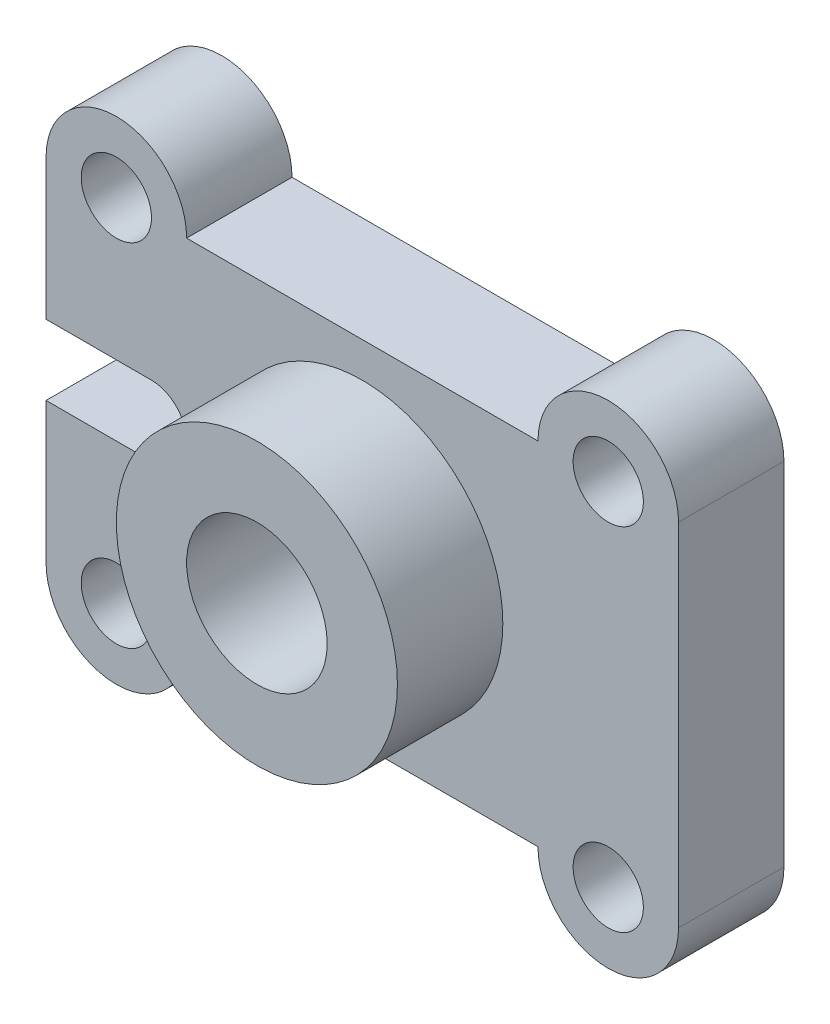
ISO-10303-21;
HEADER;
FILE_DESCRIPTION(('STEP AP214'),'2;1');
FILE_NAME('part.step','',(''),(''),'','','');
FILE_SCHEMA(('AUTOMOTIVE_DESIGN { 1 0 10303 214 1 1 1 1 }'));
ENDSEC;
DATA;
#1=APPLICATION_CONTEXT('core data for automotive mechanical design processes');
#2=APPLICATION_PROTOCOL_DEFINITION('international standard','automotive_design',2000,#1);
#3=PRODUCT_CONTEXT('',#1,'mechanical');
#4=PRODUCT('Part','Part','',(#3));
#5=PRODUCT_RELATED_PRODUCT_CATEGORY('part','',(#4));
#6=PRODUCT_DEFINITION_FORMATION('','',#4);
#7=PRODUCT_DEFINITION_CONTEXT('part definition',#1,'design');
#8=PRODUCT_DEFINITION('design','',#6,#7);
#9=PRODUCT_DEFINITION_SHAPE('','',#8);
#10=(LENGTH_UNIT() NAMED_UNIT(*) SI_UNIT(.MILLI.,.METRE.));
#11=(NAMED_UNIT(*) PLANE_ANGLE_UNIT() SI_UNIT($,.RADIAN.));
#12=(NAMED_UNIT(*) SI_UNIT($,.STERADIAN.) SOLID_ANGLE_UNIT());
#13=UNCERTAINTY_MEASURE_WITH_UNIT(LENGTH_MEASURE(1.E-05),#10,'distance_accuracy_value','');
#14=(GEOMETRIC_REPRESENTATION_CONTEXT(3) GLOBAL_UNCERTAINTY_ASSIGNED_CONTEXT((#13)) GLOBAL_UNIT_ASSIGNED_CONTEXT((#10,
#11,#12)) REPRESENTATION_CONTEXT('',''));
#15=CARTESIAN_POINT('',(0.,0.,0.));
#16=DIRECTION('',(0.,0.,1.));
#17=DIRECTION('',(1.,0.,0.));
#18=AXIS2_PLACEMENT_3D('',#15,#16,#17);
#19=CARTESIAN_POINT('',(8.92547525553978E-07,-50.0000066960144,15.));
#20=DIRECTION('',(0.,0.,-1.));
#21=DIRECTION('',(-1.,0.,0.));
#22=AXIS2_PLACEMENT_3D('',#19,#20,#21);
#23=CYLINDRICAL_SURFACE('',#22,10.0000000000001);
#24=CARTESIAN_POINT('',(8.92547525553978E-07,-50.0000066960144,0.));
#25=DIRECTION('',(0.,0.,1.));
#26=DIRECTION('',(1.,0.,0.));
#27=AXIS2_PLACEMENT_3D('',#24,#25,#26);
#28=CIRCLE('',#27,10.0000000000001);
#29=CARTESIAN_POINT('',(-9.99999910745245,-50.0000066960144,0.));
#30=VERTEX_POINT('',#29);
#31=CARTESIAN_POINT('',(10.0000008925476,-50.0000051331027,0.));
#32=VERTEX_POINT('',#31);
#33=EDGE_CURVE('E164',#30,#32,#28,.T.);
#34=ORIENTED_EDGE('',*,*,#33,.T.);
#35=DIRECTION('',(0.,0.,-1.));
#36=VECTOR('',#35,1.);
#37=CARTESIAN_POINT('',(10.0000008925476,-50.0000051331027,15.));
#38=LINE('',#37,#36);
#39=CARTESIAN_POINT('',(10.0000008925476,-50.0000051331027,15.));
#40=VERTEX_POINT('',#39);
#41=EDGE_CURVE('E11',#40,#32,#38,.T.);
#42=ORIENTED_EDGE('',*,*,#41,.F.);
#43=CARTESIAN_POINT('',(8.92547525553978E-07,-50.0000066960144,15.));
#44=DIRECTION('',(0.,0.,1.));
#45=DIRECTION('',(1.,0.,0.));
#46=AXIS2_PLACEMENT_3D('',#43,#44,#45);
#47=CIRCLE('',#46,10.0000000000001);
#48=CARTESIAN_POINT('',(-9.99999910745245,-50.0000066960144,15.));
#49=VERTEX_POINT('',#48);
#50=EDGE_CURVE('E186',#49,#40,#47,.T.);
#51=ORIENTED_EDGE('',*,*,#50,.F.);
#52=DIRECTION('',(0.,0.,-1.));
#53=VECTOR('',#52,1.);
#54=CARTESIAN_POINT('',(-9.99999910745245,-50.0000066960144,15.));
#55=LINE('',#54,#53);
#56=EDGE_CURVE('E161',#49,#30,#55,.T.);
#57=ORIENTED_EDGE('',*,*,#56,.T.);
#58=EDGE_LOOP('',(#34,#42,#51,#57));
#59=FACE_BOUND('',#58,.T.);
#60=ADVANCED_FACE('F44',(#59),#23,.T.);
#61=CARTESIAN_POINT('',(59.9999991074522,-50.0000051331027,15.));
#62=DIRECTION('',(0.,1.,0.));
#63=DIRECTION('',(-1.,0.,0.));
#64=AXIS2_PLACEMENT_3D('',#61,#62,#63);
#65=PLANE('',#64);
#66=DIRECTION('',(1.,0.,0.));
#67=VECTOR('',#66,1.);
#68=CARTESIAN_POINT('',(59.9999991074522,-50.0000051331027,0.));
#69=LINE('',#68,#67);
#70=CARTESIAN_POINT('',(59.9999991074522,-50.0000051331027,0.));
#71=VERTEX_POINT('',#70);
#72=EDGE_CURVE('E169',#32,#71,#69,.T.);
#73=ORIENTED_EDGE('',*,*,#72,.T.);
#74=DIRECTION('',(0.,0.,-1.));
#75=VECTOR('',#74,1.);
#76=CARTESIAN_POINT('',(59.9999991074522,-50.0000051331027,15.));
#77=LINE('',#76,#75);
#78=CARTESIAN_POINT('',(59.9999991074522,-50.0000051331027,15.));
#79=VERTEX_POINT('',#78);
#80=EDGE_CURVE('E52',#79,#71,#77,.T.);
#81=ORIENTED_EDGE('',*,*,#80,.F.);
#82=DIRECTION('',(1.,0.,0.));
#83=VECTOR('',#82,1.);
#84=CARTESIAN_POINT('',(59.9999991074522,-50.0000051331027,15.));
#85=LINE('',#84,#83);
#86=EDGE_CURVE('E118',#40,#79,#85,.T.);
#87=ORIENTED_EDGE('',*,*,#86,.F.);
#88=ORIENTED_EDGE('',*,*,#41,.T.);
#89=EDGE_LOOP('',(#73,#81,#87,#88));
#90=FACE_BOUND('',#89,.T.);
#91=ADVANCED_FACE('F267',(#90),#65,.F.);
#92=CARTESIAN_POINT('',(69.9999991074519,-50.0000000000001,15.));
#93=DIRECTION('',(0.,0.,-1.));
#94=DIRECTION('',(-1.,0.,0.));
#95=AXIS2_PLACEMENT_3D('',#92,#93,#94);
#96=CYLINDRICAL_SURFACE('',#95,10.0000000000006);
#97=CARTESIAN_POINT('',(69.9999991074519,-50.0000000000001,0.));
#98=DIRECTION('',(0.,0.,1.));
#99=DIRECTION('',(1.,0.,0.));
#100=AXIS2_PLACEMENT_3D('',#97,#98,#99);
#101=CIRCLE('',#100,10.0000000000006);
#102=CARTESIAN_POINT('',(79.9999991074525,-50.0000000000001,0.));
#103=VERTEX_POINT('',#102);
#104=EDGE_CURVE('E173',#71,#103,#101,.T.);
#105=ORIENTED_EDGE('',*,*,#104,.T.);
#106=DIRECTION('',(0.,0.,-1.));
#107=VECTOR('',#106,1.);
#108=CARTESIAN_POINT('',(79.9999991074525,-50.0000000000001,15.));
#109=LINE('',#108,#107);
#110=CARTESIAN_POINT('',(79.9999991074525,-50.0000000000001,15.));
#111=VERTEX_POINT('',#110);
#112=EDGE_CURVE('E210',#111,#103,#109,.T.);
#113=ORIENTED_EDGE('',*,*,#112,.F.);
#114=CARTESIAN_POINT('',(69.9999991074519,-50.0000000000001,15.));
#115=DIRECTION('',(0.,0.,1.));
#116=DIRECTION('',(1.,0.,0.));
#117=AXIS2_PLACEMENT_3D('',#114,#115,#116);
#118=CIRCLE('',#117,10.0000000000006);
#119=EDGE_CURVE('E214',#79,#111,#118,.T.);
#120=ORIENTED_EDGE('',*,*,#119,.F.);
#121=ORIENTED_EDGE('',*,*,#80,.T.);
#122=EDGE_LOOP('',(#105,#113,#120,#121));
#123=FACE_BOUND('',#122,.T.);
#124=ADVANCED_FACE('F213',(#123),#96,.T.);
#125=CARTESIAN_POINT('',(79.999999107452,0.,15.));
#126=DIRECTION('',(-1.,0.,0.));
#127=DIRECTION('',(0.,-1.,0.));
#128=AXIS2_PLACEMENT_3D('',#125,#126,#127);
#129=PLANE('',#128);
#130=DIRECTION('',(0.,1.,0.));
#131=VECTOR('',#130,1.);
#132=CARTESIAN_POINT('',(79.999999107452,0.,0.));
#133=LINE('',#132,#131);
#134=CARTESIAN_POINT('',(79.999999107452,0.,0.));
#135=VERTEX_POINT('',#134);
#136=EDGE_CURVE('E171',#103,#135,#133,.T.);
#137=ORIENTED_EDGE('',*,*,#136,.T.);
#138=DIRECTION('',(0.,0.,-1.));
#139=VECTOR('',#138,1.);
#140=CARTESIAN_POINT('',(79.999999107452,0.,15.));
#141=LINE('',#140,#139);
#142=CARTESIAN_POINT('',(79.999999107452,0.,15.));
#143=VERTEX_POINT('',#142);
#144=EDGE_CURVE('E204',#143,#135,#141,.T.);
#145=ORIENTED_EDGE('',*,*,#144,.F.);
#146=DIRECTION('',(0.,1.,0.));
#147=VECTOR('',#146,1.);
#148=CARTESIAN_POINT('',(79.999999107452,0.,15.));
#149=LINE('',#148,#147);
#150=EDGE_CURVE('E235',#111,#143,#149,.T.);
#151=ORIENTED_EDGE('',*,*,#150,.F.);
#152=ORIENTED_EDGE('',*,*,#112,.T.);
#153=EDGE_LOOP('',(#137,#145,#151,#152));
#154=FACE_BOUND('',#153,.T.);
#155=ADVANCED_FACE('F221',(#154),#129,.F.);
#156=CARTESIAN_POINT('',(69.999999107452,0.,15.));
#157=DIRECTION('',(0.,0.,-1.));
#158=DIRECTION('',(-1.,0.,0.));
#159=AXIS2_PLACEMENT_3D('',#156,#157,#158);
#160=CYLINDRICAL_SURFACE('',#159,10.0000000000005);
#161=CARTESIAN_POINT('',(69.999999107452,0.,0.));
#162=DIRECTION('',(0.,0.,1.));
#163=DIRECTION('',(1.,0.,0.));
#164=AXIS2_PLACEMENT_3D('',#161,#162,#163);
#165=CIRCLE('',#164,10.0000000000005);
#166=CARTESIAN_POINT('',(59.9999991074528,-5.13310270243646E-06,0.));
#167=VERTEX_POINT('',#166);
#168=EDGE_CURVE('E172',#135,#167,#165,.T.);
#169=ORIENTED_EDGE('',*,*,#168,.T.);
#170=DIRECTION('',(0.,0.,-1.));
#171=VECTOR('',#170,1.);
#172=CARTESIAN_POINT('',(59.9999991074528,-5.13310270243646E-06,15.));
#173=LINE('',#172,#171);
#174=CARTESIAN_POINT('',(59.9999991074528,-5.13310270243646E-06,15.));
#175=VERTEX_POINT('',#174);
#176=EDGE_CURVE('E203',#175,#167,#173,.T.);
#177=ORIENTED_EDGE('',*,*,#176,.F.);
#178=CARTESIAN_POINT('',(69.999999107452,0.,15.));
#179=DIRECTION('',(0.,0.,1.));
#180=DIRECTION('',(1.,0.,0.));
#181=AXIS2_PLACEMENT_3D('',#178,#179,#180);
#182=CIRCLE('',#181,10.0000000000005);
#183=EDGE_CURVE('E227',#143,#175,#182,.T.);
#184=ORIENTED_EDGE('',*,*,#183,.F.);
#185=ORIENTED_EDGE('',*,*,#144,.T.);
#186=EDGE_LOOP('',(#169,#177,#184,#185));
#187=FACE_BOUND('',#186,.T.);
#188=ADVANCED_FACE('F226',(#187),#160,.T.);
#189=CARTESIAN_POINT('',(9.99999910745228,-5.13310270598176E-06,15.));
#190=DIRECTION('',(0.,-1.,0.));
#191=DIRECTION('',(1.,0.,0.));
#192=AXIS2_PLACEMENT_3D('',#189,#190,#191);
#193=PLANE('',#192);
#194=DIRECTION('',(-1.,0.,0.));
#195=VECTOR('',#194,1.);
#196=CARTESIAN_POINT('',(9.99999910745228,-5.13310270598176E-06,0.));
#197=LINE('',#196,#195);
#198=CARTESIAN_POINT('',(9.99999910745228,-5.13310270598176E-06,0.));
#199=VERTEX_POINT('',#198);
#200=EDGE_CURVE('E179',#167,#199,#197,.T.);
#201=ORIENTED_EDGE('',*,*,#200,.T.);
#202=DIRECTION('',(0.,0.,-1.));
#203=VECTOR('',#202,1.);
#204=CARTESIAN_POINT('',(9.99999910745228,-5.13310270598176E-06,15.));
#205=LINE('',#204,#203);
#206=CARTESIAN_POINT('',(9.99999910745228,-5.13310270598176E-06,15.));
#207=VERTEX_POINT('',#206);
#208=EDGE_CURVE('E196',#207,#199,#205,.T.);
#209=ORIENTED_EDGE('',*,*,#208,.F.);
#210=DIRECTION('',(-1.,0.,0.));
#211=VECTOR('',#210,1.);
#212=CARTESIAN_POINT('',(9.99999910745228,-5.13310270598176E-06,15.));
#213=LINE('',#212,#211);
#214=EDGE_CURVE('E234',#175,#207,#213,.T.);
#215=ORIENTED_EDGE('',*,*,#214,.F.);
#216=ORIENTED_EDGE('',*,*,#176,.T.);
#217=EDGE_LOOP('',(#201,#209,#215,#216));
#218=FACE_BOUND('',#217,.T.);
#219=ADVANCED_FACE('F284',(#218),#193,.F.);
#220=CARTESIAN_POINT('',(0.,0.,15.));
#221=DIRECTION('',(0.,0.,-1.));
#222=DIRECTION('',(-1.,0.,0.));
#223=AXIS2_PLACEMENT_3D('',#220,#221,#222);
#224=CYLINDRICAL_SURFACE('',#223,9.99999910745303);
#225=CARTESIAN_POINT('',(0.,0.,0.));
#226=DIRECTION('',(0.,0.,1.));
#227=DIRECTION('',(1.,0.,0.));
#228=AXIS2_PLACEMENT_3D('',#225,#226,#227);
#229=CIRCLE('',#228,9.99999910745303);
#230=CARTESIAN_POINT('',(-9.99999910745303,0.,0.));
#231=VERTEX_POINT('',#230);
#232=EDGE_CURVE('E176',#199,#231,#229,.T.);
#233=ORIENTED_EDGE('',*,*,#232,.T.);
#234=DIRECTION('',(0.,0.,-1.));
#235=VECTOR('',#234,1.);
#236=CARTESIAN_POINT('',(-9.99999910745303,0.,15.));
#237=LINE('',#236,#235);
#238=CARTESIAN_POINT('',(-9.99999910745303,0.,15.));
#239=VERTEX_POINT('',#238);
#240=EDGE_CURVE('E193',#239,#231,#237,.T.);
#241=ORIENTED_EDGE('',*,*,#240,.F.);
#242=CARTESIAN_POINT('',(0.,0.,15.));
#243=DIRECTION('',(0.,0.,1.));
#244=DIRECTION('',(1.,0.,0.));
#245=AXIS2_PLACEMENT_3D('',#242,#243,#244);
#246=CIRCLE('',#245,9.99999910745303);
#247=EDGE_CURVE('E233',#207,#239,#246,.T.);
#248=ORIENTED_EDGE('',*,*,#247,.F.);
#249=ORIENTED_EDGE('',*,*,#208,.T.);
#250=EDGE_LOOP('',(#233,#241,#248,#249));
#251=FACE_BOUND('',#250,.T.);
#252=ADVANCED_FACE('F289',(#251),#224,.T.);
#253=CARTESIAN_POINT('',(-9.99999910745246,0.,15.));
#254=DIRECTION('',(1.,0.,0.));
#255=DIRECTION('',(0.,1.,0.));
#256=AXIS2_PLACEMENT_3D('',#253,#254,#255);
#257=PLANE('',#256);
#258=DIRECTION('',(0.,-1.,0.));
#259=VECTOR('',#258,1.);
#260=CARTESIAN_POINT('',(-9.99999910745246,0.,0.));
#261=LINE('',#260,#259);
#262=CARTESIAN_POINT('',(-9.99999910745245,-20.,0.));
#263=VERTEX_POINT('',#262);
#264=EDGE_CURVE('E182',#231,#263,#261,.T.);
#265=ORIENTED_EDGE('',*,*,#264,.T.);
#266=DIRECTION('',(0.,0.,-1.));
#267=VECTOR('',#266,1.);
#268=CARTESIAN_POINT('',(-9.99999910745245,-20.,15.));
#269=LINE('',#268,#267);
#270=CARTESIAN_POINT('',(-9.99999910745245,-20.,15.));
#271=VERTEX_POINT('',#270);
#272=EDGE_CURVE('E194',#271,#263,#269,.T.);
#273=ORIENTED_EDGE('',*,*,#272,.F.);
#274=DIRECTION('',(0.,-1.,0.));
#275=VECTOR('',#274,1.);
#276=CARTESIAN_POINT('',(-9.99999910745246,0.,15.));
#277=LINE('',#276,#275);
#278=EDGE_CURVE('E243',#239,#271,#277,.T.);
#279=ORIENTED_EDGE('',*,*,#278,.F.);
#280=ORIENTED_EDGE('',*,*,#240,.T.);
#281=EDGE_LOOP('',(#265,#273,#279,#280));
#282=FACE_BOUND('',#281,.T.);
#283=ADVANCED_FACE('F249',(#282),#257,.F.);
#284=CARTESIAN_POINT('',(-9.99999910745245,-20.,15.));
#285=DIRECTION('',(0.,1.,0.));
#286=DIRECTION('',(-1.,0.,0.));
#287=AXIS2_PLACEMENT_3D('',#284,#285,#286);
#288=PLANE('',#287);
#289=DIRECTION('',(1.,0.,0.));
#290=VECTOR('',#289,1.);
#291=CARTESIAN_POINT('',(-9.99999910745245,-20.,0.));
#292=LINE('',#291,#290);
#293=CARTESIAN_POINT('',(5.00000267764276,-20.,0.));
#294=VERTEX_POINT('',#293);
#295=EDGE_CURVE('E181',#263,#294,#292,.T.);
#296=ORIENTED_EDGE('',*,*,#295,.T.);
#297=DIRECTION('',(0.,0.,-1.));
#298=VECTOR('',#297,1.);
#299=CARTESIAN_POINT('',(5.00000267764276,-20.,15.));
#300=LINE('',#299,#298);
#301=CARTESIAN_POINT('',(5.00000267764276,-20.,15.));
#302=VERTEX_POINT('',#301);
#303=EDGE_CURVE('E156',#302,#294,#300,.T.);
#304=ORIENTED_EDGE('',*,*,#303,.F.);
#305=DIRECTION('',(1.,0.,0.));
#306=VECTOR('',#305,1.);
#307=CARTESIAN_POINT('',(-9.99999910745245,-20.,15.));
#308=LINE('',#307,#306);
#309=EDGE_CURVE('E150',#271,#302,#308,.T.);
#310=ORIENTED_EDGE('',*,*,#309,.F.);
#311=ORIENTED_EDGE('',*,*,#272,.T.);
#312=EDGE_LOOP('',(#296,#304,#310,#311));
#313=FACE_BOUND('',#312,.T.);
#314=ADVANCED_FACE('F253',(#313),#288,.F.);
#315=CARTESIAN_POINT('',(5.00000169147834,-25.,15.));
#316=DIRECTION('',(0.,0.,-1.));
#317=DIRECTION('',(-1.,0.,0.));
#318=AXIS2_PLACEMENT_3D('',#315,#316,#317);
#319=CYLINDRICAL_SURFACE('',#318,5.00000000000008);
#320=CARTESIAN_POINT('',(5.00000169147834,-25.,0.));
#321=DIRECTION('',(0.,0.,-1.));
#322=DIRECTION('',(1.,0.,0.));
#323=AXIS2_PLACEMENT_3D('',#320,#321,#322);
#324=CIRCLE('',#323,5.00000000000008);
#325=CARTESIAN_POINT('',(5.00000089254754,-30.0000000000001,0.));
#326=VERTEX_POINT('',#325);
#327=EDGE_CURVE('E154',#294,#326,#324,.T.);
#328=ORIENTED_EDGE('',*,*,#327,.T.);
#329=DIRECTION('',(0.,0.,-1.));
#330=VECTOR('',#329,1.);
#331=CARTESIAN_POINT('',(5.00000089254754,-30.0000000000001,15.));
#332=LINE('',#331,#330);
#333=CARTESIAN_POINT('',(5.00000089254754,-30.0000000000001,15.));
#334=VERTEX_POINT('',#333);
#335=EDGE_CURVE('E155',#334,#326,#332,.T.);
#336=ORIENTED_EDGE('',*,*,#335,.F.);
#337=CARTESIAN_POINT('',(5.00000169147834,-25.,15.));
#338=DIRECTION('',(0.,0.,-1.));
#339=DIRECTION('',(1.,0.,0.));
#340=AXIS2_PLACEMENT_3D('',#337,#338,#339);
#341=CIRCLE('',#340,5.00000000000008);
#342=EDGE_CURVE('E143',#302,#334,#341,.T.);
#343=ORIENTED_EDGE('',*,*,#342,.F.);
#344=ORIENTED_EDGE('',*,*,#303,.T.);
#345=EDGE_LOOP('',(#328,#336,#343,#344));
#346=FACE_BOUND('',#345,.T.);
#347=ADVANCED_FACE('F153',(#346),#319,.F.);
#348=CARTESIAN_POINT('',(5.00000089254754,-30.,15.));
#349=DIRECTION('',(0.,-1.,0.));
#350=DIRECTION('',(1.,0.,0.));
#351=AXIS2_PLACEMENT_3D('',#348,#349,#350);
#352=PLANE('',#351);
#353=DIRECTION('',(-1.,0.,0.));
#354=VECTOR('',#353,1.);
#355=CARTESIAN_POINT('',(5.00000089254754,-30.,0.));
#356=LINE('',#355,#354);
#357=CARTESIAN_POINT('',(-9.99999910745245,-30.,0.));
#358=VERTEX_POINT('',#357);
#359=EDGE_CURVE('E105',#326,#358,#356,.T.);
#360=ORIENTED_EDGE('',*,*,#359,.T.);
#361=DIRECTION('',(0.,0.,-1.));
#362=VECTOR('',#361,1.);
#363=CARTESIAN_POINT('',(-9.99999910745245,-30.,15.));
#364=LINE('',#363,#362);
#365=CARTESIAN_POINT('',(-9.99999910745245,-30.,15.));
#366=VERTEX_POINT('',#365);
#367=EDGE_CURVE('E160',#366,#358,#364,.T.);
#368=ORIENTED_EDGE('',*,*,#367,.F.);
#369=DIRECTION('',(-1.,0.,0.));
#370=VECTOR('',#369,1.);
#371=CARTESIAN_POINT('',(5.00000089254754,-30.,15.));
#372=LINE('',#371,#370);
#373=EDGE_CURVE('E144',#334,#366,#372,.T.);
#374=ORIENTED_EDGE('',*,*,#373,.F.);
#375=ORIENTED_EDGE('',*,*,#335,.T.);
#376=EDGE_LOOP('',(#360,#368,#374,#375));
#377=FACE_BOUND('',#376,.T.);
#378=ADVANCED_FACE('F157',(#377),#352,.F.);
#379=CARTESIAN_POINT('',(-9.99999910745245,-30.,15.));
#380=DIRECTION('',(1.,0.,0.));
#381=DIRECTION('',(0.,1.,0.));
#382=AXIS2_PLACEMENT_3D('',#379,#380,#381);
#383=PLANE('',#382);
#384=DIRECTION('',(0.,-1.,0.));
#385=VECTOR('',#384,1.);
#386=CARTESIAN_POINT('',(-9.99999910745245,-30.,0.));
#387=LINE('',#386,#385);
#388=EDGE_CURVE('E107',#358,#30,#387,.T.);
#389=ORIENTED_EDGE('',*,*,#388,.T.);
#390=ORIENTED_EDGE('',*,*,#56,.F.);
#391=DIRECTION('',(0.,-1.,0.));
#392=VECTOR('',#391,1.);
#393=CARTESIAN_POINT('',(-9.99999910745245,-30.,15.));
#394=LINE('',#393,#392);
#395=EDGE_CURVE('E63',#366,#49,#394,.T.);
#396=ORIENTED_EDGE('',*,*,#395,.F.);
#397=ORIENTED_EDGE('',*,*,#367,.T.);
#398=EDGE_LOOP('',(#389,#390,#396,#397));
#399=FACE_BOUND('',#398,.T.);
#400=ADVANCED_FACE('F254',(#399),#383,.F.);
#401=CARTESIAN_POINT('',(8.92547525553978E-07,-50.0000066960144,15.));
#402=DIRECTION('',(0.,0.,1.));
#403=DIRECTION('',(1.,0.,0.));
#404=AXIS2_PLACEMENT_3D('',#401,#402,#403);
#405=PLANE('',#404);
#406=CARTESIAN_POINT('',(34.9999991074525,-25.0000051331027,15.));
#407=DIRECTION('',(0.,0.,1.));
#408=DIRECTION('',(1.,0.,0.));
#409=AXIS2_PLACEMENT_3D('',#406,#407,#408);
#410=CIRCLE('',#409,20.);
#411=CARTESIAN_POINT('',(54.9999991074525,-25.0000051331027,15.));
#412=VERTEX_POINT('',#411);
#413=EDGE_CURVE('E567',#412,#412,#410,.T.);
#414=ORIENTED_EDGE('',*,*,#413,.F.);
#415=EDGE_LOOP('',(#414));
#416=FACE_BOUND('',#415,.T.);
#417=CARTESIAN_POINT('',(8.92547525553978E-07,-50.0000066960144,15.));
#418=DIRECTION('',(0.,0.,1.));
#419=DIRECTION('',(1.,0.,0.));
#420=AXIS2_PLACEMENT_3D('',#417,#418,#419);
#421=CIRCLE('',#420,5.00000000000001);
#422=CARTESIAN_POINT('',(5.00000089254753,-50.0000066960144,15.));
#423=VERTEX_POINT('',#422);
#424=EDGE_CURVE('E552',#423,#423,#421,.T.);
#425=ORIENTED_EDGE('',*,*,#424,.F.);
#426=EDGE_LOOP('',(#425));
#427=FACE_BOUND('',#426,.T.);
#428=CARTESIAN_POINT('',(69.9999991074519,-50.0000000000001,15.));
#429=DIRECTION('',(0.,0.,1.));
#430=DIRECTION('',(1.,0.,0.));
#431=AXIS2_PLACEMENT_3D('',#428,#429,#430);
#432=CIRCLE('',#431,5.00000000000001);
#433=CARTESIAN_POINT('',(74.9999991074519,-50.0000000000001,15.));
#434=VERTEX_POINT('',#433);
#435=EDGE_CURVE('E556',#434,#434,#432,.T.);
#436=ORIENTED_EDGE('',*,*,#435,.F.);
#437=EDGE_LOOP('',(#436));
#438=FACE_BOUND('',#437,.T.);
#439=CARTESIAN_POINT('',(69.999999107452,0.,15.));
#440=DIRECTION('',(0.,0.,1.));
#441=DIRECTION('',(1.,0.,0.));
#442=AXIS2_PLACEMENT_3D('',#439,#440,#441);
#443=CIRCLE('',#442,5.);
#444=CARTESIAN_POINT('',(74.999999107452,0.,15.));
#445=VERTEX_POINT('',#444);
#446=EDGE_CURVE('E564',#445,#445,#443,.T.);
#447=ORIENTED_EDGE('',*,*,#446,.F.);
#448=EDGE_LOOP('',(#447));
#449=FACE_BOUND('',#448,.T.);
#450=CARTESIAN_POINT('',(0.,0.,15.));
#451=DIRECTION('',(0.,0.,1.));
#452=DIRECTION('',(1.,0.,0.));
#453=AXIS2_PLACEMENT_3D('',#450,#451,#452);
#454=CIRCLE('',#453,5.);
#455=CARTESIAN_POINT('',(5.,0.,15.));
#456=VERTEX_POINT('',#455);
#457=EDGE_CURVE('E546',#456,#456,#454,.T.);
#458=ORIENTED_EDGE('',*,*,#457,.F.);
#459=EDGE_LOOP('',(#458));
#460=FACE_BOUND('',#459,.T.);
#461=ORIENTED_EDGE('',*,*,#50,.T.);
#462=ORIENTED_EDGE('',*,*,#86,.T.);
#463=ORIENTED_EDGE('',*,*,#119,.T.);
#464=ORIENTED_EDGE('',*,*,#150,.T.);
#465=ORIENTED_EDGE('',*,*,#183,.T.);
#466=ORIENTED_EDGE('',*,*,#214,.T.);
#467=ORIENTED_EDGE('',*,*,#247,.T.);
#468=ORIENTED_EDGE('',*,*,#278,.T.);
#469=ORIENTED_EDGE('',*,*,#309,.T.);
#470=ORIENTED_EDGE('',*,*,#342,.T.);
#471=ORIENTED_EDGE('',*,*,#373,.T.);
#472=ORIENTED_EDGE('',*,*,#395,.T.);
#473=EDGE_LOOP('',(#461,#462,#463,#464,#465,#466,#467,#468,#469,#470,#471,#472));
#474=FACE_BOUND('',#473,.T.);
#475=ADVANCED_FACE('F141',(#416,#427,#438,#449,#460,#474),#405,.T.);
#476=CARTESIAN_POINT('',(8.92547525553978E-07,-50.0000066960144,0.));
#477=DIRECTION('',(0.,0.,1.));
#478=DIRECTION('',(1.,0.,0.));
#479=AXIS2_PLACEMENT_3D('',#476,#477,#478);
#480=PLANE('',#479);
#481=CARTESIAN_POINT('',(8.92547525553978E-07,-50.0000066960144,0.));
#482=DIRECTION('',(0.,0.,1.));
#483=DIRECTION('',(1.,0.,0.));
#484=AXIS2_PLACEMENT_3D('',#481,#482,#483);
#485=CIRCLE('',#484,5.00000000000001);
#486=CARTESIAN_POINT('',(5.00000089254753,-50.0000066960144,0.));
#487=VERTEX_POINT('',#486);
#488=EDGE_CURVE('E532',#487,#487,#485,.T.);
#489=ORIENTED_EDGE('',*,*,#488,.T.);
#490=EDGE_LOOP('',(#489));
#491=FACE_BOUND('',#490,.T.);
#492=CARTESIAN_POINT('',(69.9999991074519,-50.0000000000001,0.));
#493=DIRECTION('',(0.,0.,1.));
#494=DIRECTION('',(1.,0.,0.));
#495=AXIS2_PLACEMENT_3D('',#492,#493,#494);
#496=CIRCLE('',#495,5.00000000000001);
#497=CARTESIAN_POINT('',(74.9999991074519,-50.0000000000001,0.));
#498=VERTEX_POINT('',#497);
#499=EDGE_CURVE('E537',#498,#498,#496,.T.);
#500=ORIENTED_EDGE('',*,*,#499,.T.);
#501=EDGE_LOOP('',(#500));
#502=FACE_BOUND('',#501,.T.);
#503=CARTESIAN_POINT('',(69.999999107452,0.,0.));
#504=DIRECTION('',(0.,0.,1.));
#505=DIRECTION('',(1.,0.,0.));
#506=AXIS2_PLACEMENT_3D('',#503,#504,#505);
#507=CIRCLE('',#506,5.);
#508=CARTESIAN_POINT('',(74.999999107452,0.,0.));
#509=VERTEX_POINT('',#508);
#510=EDGE_CURVE('E543',#509,#509,#507,.T.);
#511=ORIENTED_EDGE('',*,*,#510,.T.);
#512=EDGE_LOOP('',(#511));
#513=FACE_BOUND('',#512,.T.);
#514=CARTESIAN_POINT('',(0.,0.,0.));
#515=DIRECTION('',(0.,0.,1.));
#516=DIRECTION('',(1.,0.,0.));
#517=AXIS2_PLACEMENT_3D('',#514,#515,#516);
#518=CIRCLE('',#517,5.);
#519=CARTESIAN_POINT('',(5.,0.,0.));
#520=VERTEX_POINT('',#519);
#521=EDGE_CURVE('E166',#520,#520,#518,.T.);
#522=ORIENTED_EDGE('',*,*,#521,.T.);
#523=EDGE_LOOP('',(#522));
#524=FACE_BOUND('',#523,.T.);
#525=ORIENTED_EDGE('',*,*,#33,.F.);
#526=ORIENTED_EDGE('',*,*,#388,.F.);
#527=ORIENTED_EDGE('',*,*,#359,.F.);
#528=ORIENTED_EDGE('',*,*,#327,.F.);
#529=ORIENTED_EDGE('',*,*,#295,.F.);
#530=ORIENTED_EDGE('',*,*,#264,.F.);
#531=ORIENTED_EDGE('',*,*,#232,.F.);
#532=ORIENTED_EDGE('',*,*,#200,.F.);
#533=ORIENTED_EDGE('',*,*,#168,.F.);
#534=ORIENTED_EDGE('',*,*,#136,.F.);
#535=ORIENTED_EDGE('',*,*,#104,.F.);
#536=ORIENTED_EDGE('',*,*,#72,.F.);
#537=EDGE_LOOP('',(#525,#526,#527,#528,#529,#530,#531,#532,#533,#534,#535,#536));
#538=FACE_BOUND('',#537,.T.);
#539=ADVANCED_FACE('F218',(#491,#502,#513,#524,#538),#480,.F.);
#540=CARTESIAN_POINT('',(0.,0.,0.));
#541=DIRECTION('',(0.,0.,1.));
#542=DIRECTION('',(1.,0.,0.));
#543=AXIS2_PLACEMENT_3D('',#540,#541,#542);
#544=CYLINDRICAL_SURFACE('',#543,5.);
#545=ORIENTED_EDGE('',*,*,#521,.F.);
#546=EDGE_LOOP('',(#545));
#547=FACE_BOUND('',#546,.T.);
#548=ORIENTED_EDGE('',*,*,#457,.T.);
#549=EDGE_LOOP('',(#548));
#550=FACE_BOUND('',#549,.T.);
#551=ADVANCED_FACE('F310',(#547,#550),#544,.F.);
#552=CARTESIAN_POINT('',(69.999999107452,0.,0.));
#553=DIRECTION('',(0.,0.,1.));
#554=DIRECTION('',(1.,0.,0.));
#555=AXIS2_PLACEMENT_3D('',#552,#553,#554);
#556=CYLINDRICAL_SURFACE('',#555,5.);
#557=ORIENTED_EDGE('',*,*,#510,.F.);
#558=EDGE_LOOP('',(#557));
#559=FACE_BOUND('',#558,.T.);
#560=ORIENTED_EDGE('',*,*,#446,.T.);
#561=EDGE_LOOP('',(#560));
#562=FACE_BOUND('',#561,.T.);
#563=ADVANCED_FACE('F315',(#559,#562),#556,.F.);
#564=CARTESIAN_POINT('',(69.9999991074519,-50.0000000000001,0.));
#565=DIRECTION('',(0.,0.,1.));
#566=DIRECTION('',(1.,0.,0.));
#567=AXIS2_PLACEMENT_3D('',#564,#565,#566);
#568=CYLINDRICAL_SURFACE('',#567,5.00000000000001);
#569=ORIENTED_EDGE('',*,*,#499,.F.);
#570=EDGE_LOOP('',(#569));
#571=FACE_BOUND('',#570,.T.);
#572=ORIENTED_EDGE('',*,*,#435,.T.);
#573=EDGE_LOOP('',(#572));
#574=FACE_BOUND('',#573,.T.);
#575=ADVANCED_FACE('F319',(#571,#574),#568,.F.);
#576=CARTESIAN_POINT('',(8.92547525553978E-07,-50.0000066960144,0.));
#577=DIRECTION('',(0.,0.,1.));
#578=DIRECTION('',(1.,0.,0.));
#579=AXIS2_PLACEMENT_3D('',#576,#577,#578);
#580=CYLINDRICAL_SURFACE('',#579,5.00000000000001);
#581=ORIENTED_EDGE('',*,*,#488,.F.);
#582=EDGE_LOOP('',(#581));
#583=FACE_BOUND('',#582,.T.);
#584=ORIENTED_EDGE('',*,*,#424,.T.);
#585=EDGE_LOOP('',(#584));
#586=FACE_BOUND('',#585,.T.);
#587=ADVANCED_FACE('F327',(#583,#586),#580,.F.);
#588=CARTESIAN_POINT('',(34.9999991074525,-25.0000051331027,30.));
#589=DIRECTION('',(0.,0.,-1.));
#590=DIRECTION('',(-1.,0.,0.));
#591=AXIS2_PLACEMENT_3D('',#588,#589,#590);
#592=CYLINDRICAL_SURFACE('',#591,20.);
#593=CARTESIAN_POINT('',(34.9999991074525,-25.0000051331027,30.));
#594=DIRECTION('',(0.,0.,1.));
#595=DIRECTION('',(1.,0.,0.));
#596=AXIS2_PLACEMENT_3D('',#593,#594,#595);
#597=CIRCLE('',#596,20.);
#598=CARTESIAN_POINT('',(54.9999991074525,-25.0000051331027,30.));
#599=VERTEX_POINT('',#598);
#600=EDGE_CURVE('E558',#599,#599,#597,.T.);
#601=ORIENTED_EDGE('',*,*,#600,.F.);
#602=EDGE_LOOP('',(#601));
#603=FACE_BOUND('',#602,.T.);
#604=ORIENTED_EDGE('',*,*,#413,.T.);
#605=EDGE_LOOP('',(#604));
#606=FACE_BOUND('',#605,.T.);
#607=ADVANCED_FACE('F338',(#603,#606),#592,.T.);
#608=CARTESIAN_POINT('',(34.9999991074525,-25.0000051331027,30.));
#609=DIRECTION('',(0.,0.,1.));
#610=DIRECTION('',(1.,0.,0.));
#611=AXIS2_PLACEMENT_3D('',#608,#609,#610);
#612=PLANE('',#611);
#613=CARTESIAN_POINT('',(34.9999991074525,-25.0000051331027,30.));
#614=DIRECTION('',(0.,0.,1.));
#615=DIRECTION('',(1.,0.,0.));
#616=AXIS2_PLACEMENT_3D('',#613,#614,#615);
#617=CIRCLE('',#616,10.);
#618=CARTESIAN_POINT('',(44.9999991074525,-25.0000051331027,30.));
#619=VERTEX_POINT('',#618);
#620=EDGE_CURVE('E575',#619,#619,#617,.T.);
#621=ORIENTED_EDGE('',*,*,#620,.F.);
#622=EDGE_LOOP('',(#621));
#623=FACE_BOUND('',#622,.T.);
#624=ORIENTED_EDGE('',*,*,#600,.T.);
#625=EDGE_LOOP('',(#624));
#626=FACE_BOUND('',#625,.T.);
#627=ADVANCED_FACE('F341',(#623,#626),#612,.T.);
#628=CARTESIAN_POINT('',(34.9999991074525,-25.0000051331027,15.));
#629=DIRECTION('',(0.,0.,1.));
#630=DIRECTION('',(1.,0.,0.));
#631=AXIS2_PLACEMENT_3D('',#628,#629,#630);
#632=CYLINDRICAL_SURFACE('',#631,10.);
#633=CARTESIAN_POINT('',(34.9999991074525,-25.0000051331027,15.));
#634=DIRECTION('',(0.,0.,1.));
#635=DIRECTION('',(1.,0.,0.));
#636=AXIS2_PLACEMENT_3D('',#633,#634,#635);
#637=CIRCLE('',#636,10.);
#638=CARTESIAN_POINT('',(44.9999991074525,-25.0000051331027,15.));
#639=VERTEX_POINT('',#638);
#640=EDGE_CURVE('E569',#639,#639,#637,.T.);
#641=ORIENTED_EDGE('',*,*,#640,.F.);
#642=EDGE_LOOP('',(#641));
#643=FACE_BOUND('',#642,.T.);
#644=ORIENTED_EDGE('',*,*,#620,.T.);
#645=EDGE_LOOP('',(#644));
#646=FACE_BOUND('',#645,.T.);
#647=ADVANCED_FACE('F355',(#643,#646),#632,.F.);
#648=CARTESIAN_POINT('',(34.9999991074525,-25.0000051331027,15.));
#649=DIRECTION('',(0.,0.,1.));
#650=DIRECTION('',(1.,0.,0.));
#651=AXIS2_PLACEMENT_3D('',#648,#649,#650);
#652=PLANE('',#651);
#653=ORIENTED_EDGE('',*,*,#640,.T.);
#654=EDGE_LOOP('',(#653));
#655=FACE_BOUND('',#654,.T.);
#656=ADVANCED_FACE('F358',(#655),#652,.T.);
#657=CLOSED_SHELL('',(#60,#91,#124,#155,#188,#219,#252,#283,#314,#347,#378,#400,#475,#539,#551,
#563,#575,#587,#607,#627,#647,#656));
#658=MANIFOLD_SOLID_BREP('B2',#657);
#659=ADVANCED_BREP_SHAPE_REPRESENTATION('',(#18,#658),#14);
#660=SHAPE_DEFINITION_REPRESENTATION(#9,#659);
ENDSEC;
END-ISO-10303-21;
